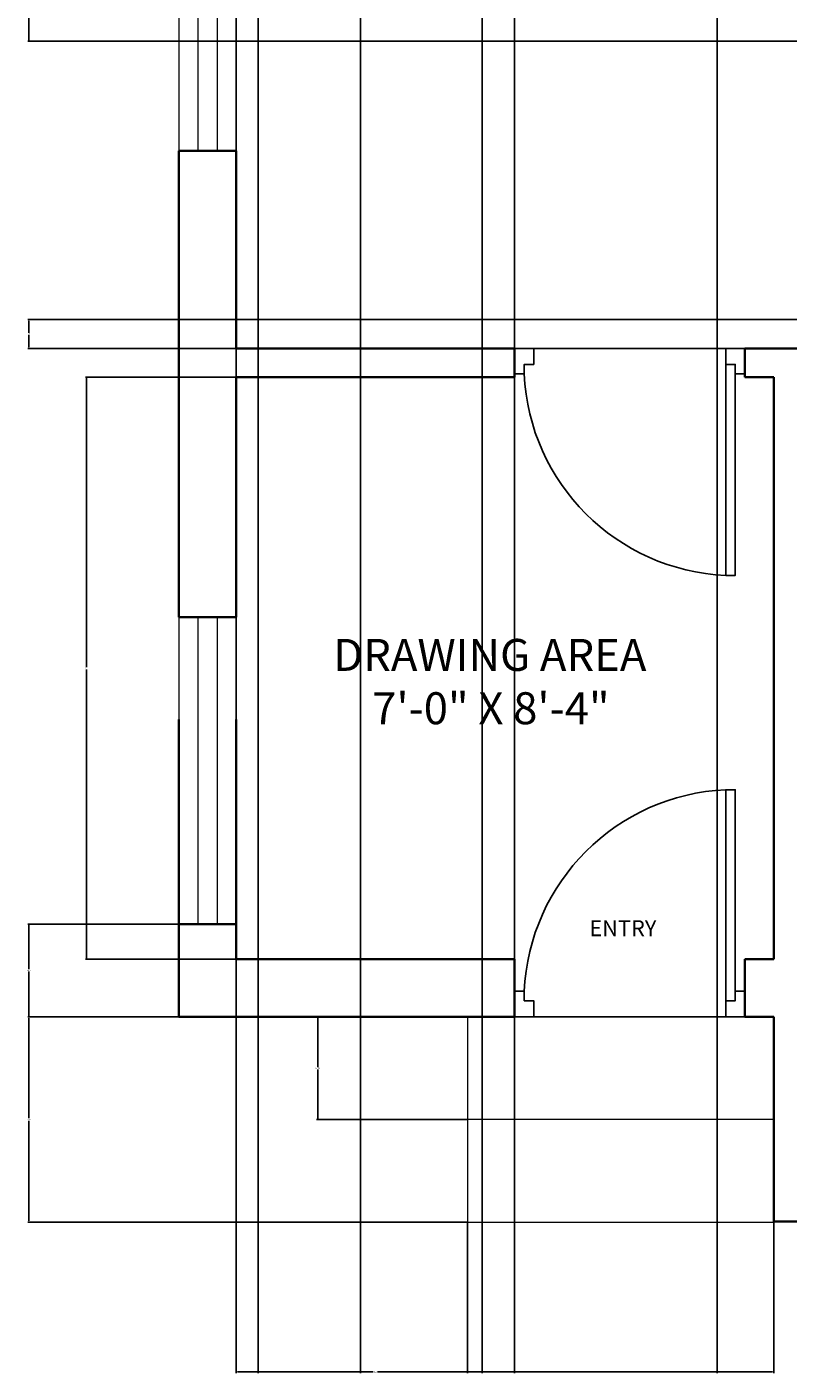
# Model space of a CAD drawing. Units: inches. Extents: x 324 to 662, y 102 to 605.
# Tile 1 of 4: x 324 to 443, y 102 to 313. Entities that reach past the tile are written whole.
import ezdxf

# ---------------------------------------------------------------- set-up
doc = ezdxf.new("R2010")
doc.units = ezdxf.units.IN
for name, color, linetype, lineweight in [('A-ANNO-DIMS', 2, 'Continuous', 18), ('A-ANNO-TEXT', 7, 'Continuous', 18), ('A-AREA-IDEN', 7, 'Continuous', 25), ('A-FLOR-STRS', 7, 'Continuous', 18), ('door', 82, 'Continuous', 25), ('wall', 7, 'Continuous', 35), ('window', 50, 'Continuous', 18)]:
    doc.layers.add(name, color=color, linetype=linetype, lineweight=lineweight)
doc.styles.get("Standard").update_dxf_attribs({"font": 'arial.ttf'})
doc.dimstyles.get("Standard").update_dxf_attribs({"dimtxt": 0.18, "dimasz": 0.18, "dimexe": 0.18, "dimexo": 0.0625, "dimgap": 0.09, "dimtad": 0, "dimtih": 1, "dimtoh": 1, "dimdec": 4, "dimzin": 0, "dimdsep": 46, "dimtxsty": 'Standard', "dimcen": 0.09, "dimadec": 0, "dimazin": 0, "dimtfac": 1, "dimtdec": 4, "dimtofl": 0, "dimtmove": 0, "dimatfit": 3, "dimfxl": 1, "dimtolj": 1, "dimtzin": 0, "dimarcsym": 0})

# ---------------------------------------------------------------- blocks, each defined once
blk = doc.blocks.new('w1')
at = {"layer": 'window'}
for p, q in [((719.66, 290.3), (719.66, 242.3)), ((722.66, 290.3), (722.66, 242.3))]:
    blk.add_line(p, q, dxfattribs=at)
blk.add_lwpolyline([(716.66, 242.3), (725.66, 242.3), (725.66, 290.3), (716.66, 290.3)], close=True, dxfattribs=at)
blk = doc.blocks.new('w2')
at = {"layer": 'window'}
for p, q in [((765.26, 316.2), (765.26, 280.2)), ((768.26, 316.2), (768.26, 280.2))]:
    blk.add_line(p, q, dxfattribs=at)
blk.add_lwpolyline([(762.26, 280.2), (771.26, 280.2), (771.26, 316.2), (762.26, 316.2)], close=True, dxfattribs=at)
blk = doc.blocks.new('d1')
at = {"layer": 'door'}
blk.add_line((825.6, 316.36), (861.6, 316.36), dxfattribs=at)
blk.add_lwpolyline([(827.1, 318.86), (828.6, 318.86), (828.6, 351.86), (827.1, 351.86)], close=True, dxfattribs=at)
for points in [[(828.6, 316.36), (825.6, 316.36), (825.6, 320.36), (827.1, 320.36), (827.1, 318.86), (828.6, 318.86), (828.6, 316.36)], [(858.6, 316.36), (861.6, 316.36), (861.6, 320.36), (860.1, 320.36), (860.1, 318.86), (858.6, 318.86), (858.6, 316.36)]]:
    blk.add_lwpolyline(points, dxfattribs=at)
blk.add_arc((827.1, 318.86), 33.03, 2.6026, 87.3974, dxfattribs=at)
blk = doc.blocks.new('*D31')
at = {"layer": 'A-ANNO-DIMS', "color": 0, "lineweight": -2, "transparency": 16777216}
for p, q in [((347.77, 172.36), (324.24, 172.36)), ((324.42, 172.18), (324.42, 165.29)), ((324.42, 158.04), (324.42, 164.93)), ((347.77, 157.86), (324.24, 157.86))]:
    blk.add_line(p, q, dxfattribs=at)
at = {"layer": 'A-ANNO-DIMS', "color": 0, "transparency": 16777216}
for points in [[(324.39, 172.18), (324.45, 172.18), (324.42, 172.36)], [(324.39, 158.04), (324.45, 158.04), (324.42, 157.86)]]:
    blk.add_solid(points, dxfattribs=at)
at = {"layer": 'Defpoints', "color": 0, "transparency": 16777216}
for p in [(347.83, 172.36), (324.42, 157.86), (347.83, 157.86)]:
    blk.add_point(p, dxfattribs=at)
at = {"layer": 'A-ANNO-DIMS', "color": 0, "transparency": 16777216, "insert": (324.42, 165.11), "char_height": 0.18, "attachment_point": 5}
blk.add_mtext('\\A1;14.5', dxfattribs=at)
blk = doc.blocks.new('*D34')
at = {"layer": 'A-ANNO-DIMS', "color": 0, "lineweight": -2, "transparency": 16777216}
for p, q in [((490.27, 403.36), (324.24, 403.36)), ((324.42, 403.18), (324.42, 357.04)), ((324.42, 310.54), (324.42, 356.68)), ((490.27, 310.36), (324.24, 310.36))]:
    blk.add_line(p, q, dxfattribs=at)
at = {"layer": 'A-ANNO-DIMS', "color": 0, "transparency": 16777216}
for points in [[(324.39, 403.18), (324.45, 403.18), (324.42, 403.36)], [(324.39, 310.54), (324.45, 310.54), (324.42, 310.36)]]:
    blk.add_solid(points, dxfattribs=at)
at = {"layer": 'Defpoints', "color": 0, "transparency": 16777216}
for p in [(490.33, 403.36), (324.42, 310.36), (490.33, 310.36)]:
    blk.add_point(p, dxfattribs=at)
at = {"layer": 'A-ANNO-DIMS', "color": 0, "transparency": 16777216, "insert": (324.42, 356.86), "char_height": 0.18, "attachment_point": 5}
blk.add_mtext('\\A1;93', dxfattribs=at)
blk = doc.blocks.new('*D39')
at = {"layer": 'A-ANNO-DIMS', "color": 0, "lineweight": -2, "transparency": 16777216}
for p, q in [((356.83, 166.92), (356.83, 605.45)), ((357.01, 605.27), (378.25, 605.27)), ((400.15, 605.27), (378.91, 605.27)), ((400.33, 166.92), (400.33, 605.45))]:
    blk.add_line(p, q, dxfattribs=at)
at = {"layer": 'A-ANNO-DIMS', "color": 0, "transparency": 16777216}
for points in [[(357.01, 605.3), (357.01, 605.24), (356.83, 605.27)], [(400.15, 605.3), (400.15, 605.24), (400.33, 605.27)]]:
    blk.add_solid(points, dxfattribs=at)
at = {"layer": 'Defpoints', "color": 0, "transparency": 16777216}
for p in [(400.33, 605.27), (356.83, 166.86), (400.33, 166.86)]:
    blk.add_point(p, dxfattribs=at)
at = {"layer": 'A-ANNO-DIMS', "color": 0, "transparency": 16777216, "insert": (378.58, 605.27), "char_height": 0.18, "attachment_point": 5}
blk.add_mtext('\\A1;43.5', dxfattribs=at)
blk = doc.blocks.new('*D40')
at = {"layer": 'A-ANNO-DIMS', "color": 0, "lineweight": -2, "transparency": 16777216}
for p, q in [((392.97, 125.71), (392.97, 102.17)), ((440.83, 125.71), (440.83, 102.17)), ((393.15, 102.35), (416.5, 102.35)), ((440.65, 102.35), (417.3, 102.35))]:
    blk.add_line(p, q, dxfattribs=at)
at = {"layer": 'A-ANNO-DIMS', "color": 0, "transparency": 16777216}
for points in [[(393.15, 102.38), (393.15, 102.32), (392.97, 102.35)], [(440.65, 102.38), (440.65, 102.32), (440.83, 102.35)]]:
    blk.add_solid(points, dxfattribs=at)
at = {"layer": 'Defpoints', "color": 0, "transparency": 16777216}
for p in [(392.97, 125.77), (440.83, 125.77), (440.83, 102.35)]:
    blk.add_point(p, dxfattribs=at)
at = {"layer": 'A-ANNO-DIMS', "color": 0, "transparency": 16777216, "insert": (416.9, 102.35), "char_height": 0.18, "attachment_point": 5}
blk.add_mtext('\\A1;47.86', dxfattribs=at)
blk = doc.blocks.new('*D41')
at = {"layer": 'A-ANNO-DIMS', "color": 0, "lineweight": -2, "transparency": 16777216}
for p, q in [((392.91, 157.86), (324.24, 157.86)), ((324.42, 157.68), (324.42, 142)), ((324.42, 125.95), (324.42, 141.63)), ((392.91, 125.77), (324.24, 125.77))]:
    blk.add_line(p, q, dxfattribs=at)
at = {"layer": 'A-ANNO-DIMS', "color": 0, "transparency": 16777216}
for points in [[(324.39, 157.68), (324.45, 157.68), (324.42, 157.86)], [(324.39, 125.95), (324.45, 125.95), (324.42, 125.77)]]:
    blk.add_solid(points, dxfattribs=at)
at = {"layer": 'Defpoints', "color": 0, "transparency": 16777216}
for p in [(324.42, 157.86), (392.97, 157.86), (392.97, 125.77)]:
    blk.add_point(p, dxfattribs=at)
at = {"layer": 'A-ANNO-DIMS', "color": 0, "transparency": 16777216, "insert": (324.42, 141.81), "char_height": 0.18, "attachment_point": 5}
blk.add_mtext('\\A1;32.09', dxfattribs=at)
blk = doc.blocks.new('*D48')
at = {"layer": 'A-ANNO-DIMS', "color": 0, "lineweight": -2, "transparency": 16777216}
for p, q in [((395.24, 552.3), (395.24, 102.17)), ((432.02, 552.3), (432.02, 102.17)), ((395.42, 102.35), (413.24, 102.35)), ((431.84, 102.35), (414.02, 102.35))]:
    blk.add_line(p, q, dxfattribs=at)
at = {"layer": 'A-ANNO-DIMS', "color": 0, "transparency": 16777216}
for points in [[(395.42, 102.38), (395.42, 102.32), (395.24, 102.35)], [(431.84, 102.38), (431.84, 102.32), (432.02, 102.35)]]:
    blk.add_solid(points, dxfattribs=at)
at = {"layer": 'Defpoints', "color": 0, "transparency": 16777216}
for p in [(395.24, 552.36), (432.02, 552.36), (432.02, 102.35)]:
    blk.add_point(p, dxfattribs=at)
at = {"layer": 'A-ANNO-DIMS', "color": 0, "transparency": 16777216, "insert": (413.63, 102.35), "char_height": 0.18, "attachment_point": 5}
blk.add_mtext('\\A1;36.79', dxfattribs=at)
blk = doc.blocks.new('*D51')
at = {"layer": 'A-ANNO-DIMS', "color": 0, "lineweight": -2, "transparency": 16777216}
for p, q in [((356.83, 455.8), (356.83, 102.17)), ((400.33, 455.8), (400.33, 102.17)), ((357.01, 102.35), (378.25, 102.35)), ((400.15, 102.35), (378.91, 102.35))]:
    blk.add_line(p, q, dxfattribs=at)
at = {"layer": 'A-ANNO-DIMS', "color": 0, "transparency": 16777216}
for points in [[(357.01, 102.38), (357.01, 102.32), (356.83, 102.35)], [(400.15, 102.38), (400.15, 102.32), (400.33, 102.35)]]:
    blk.add_solid(points, dxfattribs=at)
at = {"layer": 'Defpoints', "color": 0, "transparency": 16777216}
for p in [(356.83, 455.86), (400.33, 455.86), (400.33, 102.35)]:
    blk.add_point(p, dxfattribs=at)
at = {"layer": 'A-ANNO-DIMS', "color": 0, "transparency": 16777216, "insert": (378.58, 102.35), "char_height": 0.18, "attachment_point": 5}
blk.add_mtext('\\A1;43.5', dxfattribs=at)
blk = doc.blocks.new('*D54')
at = {"layer": 'A-ANNO-DIMS', "color": 0, "lineweight": -2, "transparency": 16777216}
for p, q in [((485.77, 266.86), (324.24, 266.86)), ((324.42, 266.68), (324.42, 264.79)), ((324.42, 262.54), (324.42, 264.43)), ((490.27, 262.36), (324.24, 262.36))]:
    blk.add_line(p, q, dxfattribs=at)
at = {"layer": 'A-ANNO-DIMS', "color": 0, "transparency": 16777216}
for points in [[(324.39, 266.68), (324.45, 266.68), (324.42, 266.86)], [(324.39, 262.54), (324.45, 262.54), (324.42, 262.36)]]:
    blk.add_solid(points, dxfattribs=at)
at = {"layer": 'Defpoints', "color": 0, "transparency": 16777216}
for p in [(485.83, 266.86), (324.42, 262.36), (490.33, 262.36)]:
    blk.add_point(p, dxfattribs=at)
at = {"layer": 'A-ANNO-DIMS', "color": 0, "transparency": 16777216, "insert": (324.42, 264.61), "char_height": 0.18, "attachment_point": 5}
blk.add_mtext('\\A1;4.5', dxfattribs=at)
blk = doc.blocks.new('*D59')
at = {"layer": 'A-ANNO-DIMS', "color": 0, "lineweight": -2, "transparency": 16777216}
for p, q in [((360.27, 478.01), (360.27, 102.17)), ((376.24, 478.01), (376.24, 102.17)), ((360.45, 102.35), (367.87, 102.35)), ((376.06, 102.35), (368.64, 102.35))]:
    blk.add_line(p, q, dxfattribs=at)
at = {"layer": 'A-ANNO-DIMS', "color": 0, "transparency": 16777216}
for points in [[(360.45, 102.38), (360.45, 102.32), (360.27, 102.35)], [(376.06, 102.38), (376.06, 102.32), (376.24, 102.35)]]:
    blk.add_solid(points, dxfattribs=at)
at = {"layer": 'Defpoints', "color": 0, "transparency": 16777216}
for p in [(360.27, 478.07), (376.24, 478.07), (376.24, 102.35)]:
    blk.add_point(p, dxfattribs=at)
at = {"layer": 'A-ANNO-DIMS', "color": 0, "transparency": 16777216, "insert": (368.25, 102.35), "char_height": 0.18, "attachment_point": 5}
blk.add_mtext('\\A1;15.97', dxfattribs=at)
blk = doc.blocks.new('*D64')
at = {"layer": 'A-ANNO-DIMS', "color": 0, "lineweight": -2, "transparency": 16777216}
for p, q in [((356.77, 257.86), (333.24, 257.86)), ((333.42, 257.68), (333.42, 212.54)), ((333.42, 167.04), (333.42, 212.18)), ((356.77, 166.86), (333.24, 166.86))]:
    blk.add_line(p, q, dxfattribs=at)
at = {"layer": 'A-ANNO-DIMS', "color": 0, "transparency": 16777216}
for points in [[(333.39, 257.68), (333.45, 257.68), (333.42, 257.86)], [(333.39, 167.04), (333.45, 167.04), (333.42, 166.86)]]:
    blk.add_solid(points, dxfattribs=at)
at = {"layer": 'Defpoints', "color": 0, "transparency": 16777216}
for p in [(333.42, 257.86), (356.83, 257.86), (356.83, 166.86)]:
    blk.add_point(p, dxfattribs=at)
at = {"layer": 'A-ANNO-DIMS', "color": 0, "transparency": 16777216, "insert": (333.42, 212.36), "char_height": 0.18, "attachment_point": 5}
blk.add_mtext('\\A1;91', dxfattribs=at)
blk = doc.blocks.new('*D65')
at = {"layer": 'A-ANNO-DIMS', "color": 0, "lineweight": -2, "transparency": 16777216}
for p, q in [((392.91, 157.86), (369.38, 157.86)), ((369.56, 157.68), (369.56, 150.02)), ((369.56, 141.99), (369.56, 149.65)), ((392.91, 141.81), (369.38, 141.81))]:
    blk.add_line(p, q, dxfattribs=at)
at = {"layer": 'A-ANNO-DIMS', "color": 0, "transparency": 16777216}
for points in [[(369.53, 157.68), (369.59, 157.68), (369.56, 157.86)], [(369.53, 141.99), (369.59, 141.99), (369.56, 141.81)]]:
    blk.add_solid(points, dxfattribs=at)
at = {"layer": 'Defpoints', "color": 0, "transparency": 16777216}
for p in [(369.56, 157.86), (392.97, 157.86), (392.97, 141.81)]:
    blk.add_point(p, dxfattribs=at)
at = {"layer": 'A-ANNO-DIMS', "color": 0, "transparency": 16777216, "insert": (369.56, 149.84), "char_height": 0.18, "attachment_point": 5}
blk.add_mtext('\\A1;16.046', dxfattribs=at)

msp = doc.modelspace()

# ---------------------------------------------------------------- linework, layer by layer
at = {"layer": 'A-FLOR-STRS'}
msp.add_line((440.8304, 141.8138), (392.9731, 141.8138), dxfattribs=at)
msp.add_lwpolyline([(440.8304, 157.8598), (392.9731, 157.8598), (392.9731, 125.7677), (440.8304, 125.7677)], close=True, dxfattribs=at)
at = {"layer": 'wall'}
for p, q in [((356.8304, 293.2144), (347.8304, 293.2144)), ((347.8304, 293.2144), (347.8304, 220.3598)), ((356.8304, 293.2144), (356.8304, 262.3598)), ((400.3304, 262.3598), (356.8304, 262.3598)), ((400.3304, 262.3598), (400.3304, 257.8598)), ((449.8304, 262.3598), (436.3304, 262.3598)), ((436.3304, 262.3598), (436.3304, 257.8598)), ((356.8304, 257.8598), (356.8304, 220.3598)), ((400.3304, 257.8598), (356.8304, 257.8598)), ((440.8304, 257.8598), (436.3304, 257.8598)), ((440.8304, 257.8598), (440.8304, 166.8598)), ((356.8304, 220.3598), (347.8304, 220.3598)), ((347.8304, 204.3598), (347.8304, 157.8598)), ((356.8304, 204.3598), (356.8304, 166.8598)), ((356.8304, 172.3598), (347.8304, 172.3598)), ((356.8304, 166.8598), (400.3304, 166.8598)), ((400.3304, 166.8598), (400.3304, 157.8598)), ((436.3304, 166.8598), (436.3304, 157.8598)), ((436.3304, 166.8598), (440.8304, 166.8598)), ((347.8304, 157.8598), (400.3304, 157.8598)), ((436.3304, 157.8598), (440.8304, 157.8598)), ((440.8304, 157.8598), (440.8304, 125.8598)), ((440.8304, 125.8598), (488.0804, 125.8598))]:
    msp.add_line(p, q, dxfattribs=at)

# ---------------------------------------------------------------- block references
at = {"layer": 'door', "rotation": 180}
msp.add_blockref('d1', (1261.935, 578.7154), dxfattribs=at)
at = {"layer": 'door', "xscale": -1}
msp.add_blockref('d1', (1261.935, -158.4959), dxfattribs=at)
at = {"layer": 'window'}
for name, p in [('w2', (-414.4328, 13.0146)), ('w1', (-368.8269, -69.9448))]:
    msp.add_blockref(name, p, dxfattribs=at)

# ---------------------------------------------------------------- texts
at = {"layer": 'A-ANNO-TEXT', "insert": (412.0104, 172.9685), "char_height": 2.5, "attachment_point": 1}
msp.add_mtext_dynamic_manual_height_columns('ENTRY', width=13.429001, gutter_width=12.5, heights=[0], dxfattribs=at)
at = {"layer": 'A-AREA-IDEN', "insert": (371.9722, 216.9382), "char_height": 5, "attachment_point": 1}
msp.add_mtext_dynamic_manual_height_columns('DRAWING AREA\\P    7\'-0" X 8\'-4"', width=74.49559, gutter_width=12.5, heights=[0], dxfattribs=at)

# ---------------------------------------------------------------- dimensions: what is measured, and where the dimension line sits
at = {"layer": 'A-ANNO-DIMS'}
for base, p1, p2, override, picture, middle in [((400.3304, 605.2748), (356.8304, 166.8598), (400.3304, 166.8598), {"dimdec": 1, "dimlfac": 1, "dimrnd": 0, "dimzin": 0, "dimdsep": 46, "dimlunit": 2}, '*D39', (378.5804, 605.2748)), ((432.0233, 102.3527), (395.2356, 552.3588), (432.0233, 552.3588), {"dimdec": 2, "dimlfac": 1, "dimrnd": 0, "dimzin": 0, "dimdsep": 46, "dimlunit": 2}, '*D48', (413.6295, 102.3527)), ((376.2379, 102.3527), (360.2695, 478.07), (376.2379, 478.07), {"dimdec": 2, "dimlfac": 1, "dimrnd": 0, "dimzin": 0, "dimdsep": 46, "dimlunit": 2}, '*D59', (368.2537, 102.3527)), ((400.3304, 102.3527), (356.8304, 455.8598), (400.3304, 455.8598), {"dimdec": 1, "dimlfac": 1, "dimrnd": 0, "dimzin": 0, "dimdsep": 46, "dimlunit": 2}, '*D51', (378.5804, 102.3527)), ((440.8304, 102.3527), (392.9731, 125.7677), (440.8304, 125.7677), {"dimdec": 2, "dimlfac": 1, "dimrnd": 0, "dimzin": 0, "dimdsep": 46, "dimlunit": 2}, '*D40', (416.9017, 102.3527))]:
    dim = msp.add_linear_dim(base=base, p1=p1, p2=p2, dimstyle='Standard', override=override, dxfattribs=at)
    dim.commit()
    dim.dimension.update_dxf_attribs({"geometry": picture, "text_midpoint": middle})
for base, p1, p2, override, picture, middle in [((324.4154, 310.3598), (490.3304, 403.3598), (490.3304, 310.3598), {"dimdec": 0, "dimlfac": 1, "dimrnd": 0, "dimzin": 0, "dimdsep": 46, "dimlunit": 2}, '*D34', (324.4154, 356.8598)), ((324.4154, 262.3598), (485.8304, 266.8598), (490.3304, 262.3598), {"dimdec": 1, "dimlfac": 1, "dimrnd": 0, "dimzin": 0, "dimdsep": 46, "dimlunit": 2}, '*D54', (324.4154, 264.6098)), ((333.4154, 257.8598), (356.8304, 166.8598), (356.8304, 257.8598), {"dimdec": 0, "dimlfac": 1, "dimrnd": 0, "dimzin": 0, "dimdsep": 46, "dimlunit": 2}, '*D64', (333.4154, 212.3598)), ((324.4154, 157.8598), (347.8304, 172.3598), (347.8304, 157.8598), {"dimdec": 1, "dimlfac": 1, "dimrnd": 0, "dimzin": 0, "dimdsep": 46, "dimlunit": 2}, '*D31', (324.4154, 165.1098)), ((324.4154, 157.8598), (392.9731, 125.7677), (392.9731, 157.8598), {"dimdec": 2, "dimlfac": 1, "dimrnd": 0, "dimzin": 0, "dimdsep": 46, "dimlunit": 2}, '*D41', (324.4154, 141.8138)), ((369.5581, 157.8598), (392.9731, 141.8138), (392.9731, 157.8598), {"dimdec": 3, "dimlfac": 1, "dimrnd": 0, "dimzin": 0, "dimdsep": 46, "dimlunit": 2}, '*D65', (369.5581, 149.8368))]:
    dim = msp.add_linear_dim(base=base, p1=p1, p2=p2, angle=90, dimstyle='Standard', override=override, dxfattribs=at)
    dim.commit()
    dim.dimension.update_dxf_attribs({"geometry": picture, "text_midpoint": middle})

doc.saveas('drawing.dxf')
